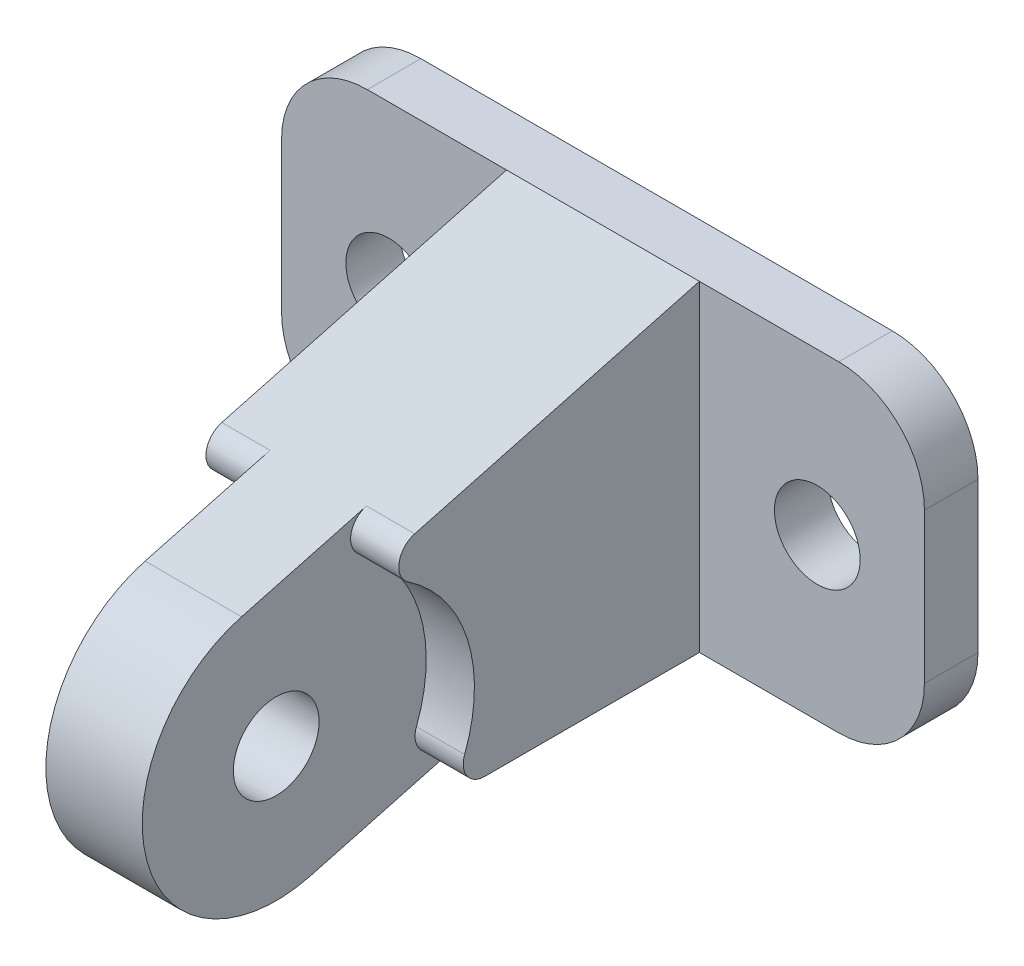
ISO-10303-21;
HEADER;
FILE_DESCRIPTION(('STEP AP214'),'2;1');
FILE_NAME('part.step','',(''),(''),'','','');
FILE_SCHEMA(('AUTOMOTIVE_DESIGN { 1 0 10303 214 1 1 1 1 }'));
ENDSEC;
DATA;
#1=APPLICATION_CONTEXT('core data for automotive mechanical design processes');
#2=APPLICATION_PROTOCOL_DEFINITION('international standard','automotive_design',2000,#1);
#3=PRODUCT_CONTEXT('',#1,'mechanical');
#4=PRODUCT('Part','Part','',(#3));
#5=PRODUCT_RELATED_PRODUCT_CATEGORY('part','',(#4));
#6=PRODUCT_DEFINITION_FORMATION('','',#4);
#7=PRODUCT_DEFINITION_CONTEXT('part definition',#1,'design');
#8=PRODUCT_DEFINITION('design','',#6,#7);
#9=PRODUCT_DEFINITION_SHAPE('','',#8);
#10=(LENGTH_UNIT() NAMED_UNIT(*) SI_UNIT(.MILLI.,.METRE.));
#11=(NAMED_UNIT(*) PLANE_ANGLE_UNIT() SI_UNIT($,.RADIAN.));
#12=(NAMED_UNIT(*) SI_UNIT($,.STERADIAN.) SOLID_ANGLE_UNIT());
#13=UNCERTAINTY_MEASURE_WITH_UNIT(LENGTH_MEASURE(1.E-05),#10,'distance_accuracy_value','');
#14=(GEOMETRIC_REPRESENTATION_CONTEXT(3) GLOBAL_UNCERTAINTY_ASSIGNED_CONTEXT((#13)) GLOBAL_UNIT_ASSIGNED_CONTEXT((#10,
#11,#12)) REPRESENTATION_CONTEXT('',''));
#15=CARTESIAN_POINT('',(0.,0.,0.));
#16=DIRECTION('',(0.,0.,1.));
#17=DIRECTION('',(1.,0.,0.));
#18=AXIS2_PLACEMENT_3D('',#15,#16,#17);
#19=CARTESIAN_POINT('',(9.,5.9476909573895,31.0562706625249));
#20=DIRECTION('',(-1.,0.,0.));
#21=DIRECTION('',(0.,0.,1.));
#22=AXIS2_PLACEMENT_3D('',#19,#20,#21);
#23=CYLINDRICAL_SURFACE('',#22,2.);
#24=CARTESIAN_POINT('',(-4.5,5.9476909573895,31.0562706625249));
#25=DIRECTION('',(1.,0.,0.));
#26=DIRECTION('',(0.,0.,-1.));
#27=AXIS2_PLACEMENT_3D('',#24,#25,#26);
#28=CIRCLE('',#27,2.);
#29=CARTESIAN_POINT('',(-4.5,7.87954260996765,31.5739087527299));
#30=VERTEX_POINT('',#29);
#31=CARTESIAN_POINT('',(-4.5,4.28933283893889,32.1742368297093));
#32=VERTEX_POINT('',#31);
#33=EDGE_CURVE('E223',#30,#32,#28,.T.);
#34=ORIENTED_EDGE('',*,*,#33,.F.);
#35=DIRECTION('',(-1.,0.,0.));
#36=VECTOR('',#35,1.);
#37=CARTESIAN_POINT('',(9.,7.87954260996765,31.5739087527299));
#38=LINE('',#37,#36);
#39=CARTESIAN_POINT('',(-9.,7.87954260996765,31.5739087527299));
#40=VERTEX_POINT('',#39);
#41=EDGE_CURVE('E292',#30,#40,#38,.T.);
#42=ORIENTED_EDGE('',*,*,#41,.T.);
#43=CARTESIAN_POINT('',(-9.,5.9476909573895,31.0562706625249));
#44=DIRECTION('',(1.,0.,0.));
#45=DIRECTION('',(0.,0.,-1.));
#46=AXIS2_PLACEMENT_3D('',#43,#44,#45);
#47=CIRCLE('',#46,2.);
#48=CARTESIAN_POINT('',(-9.,4.28933283893889,32.1742368297093));
#49=VERTEX_POINT('',#48);
#50=EDGE_CURVE('E264',#40,#49,#47,.T.);
#51=ORIENTED_EDGE('',*,*,#50,.T.);
#52=DIRECTION('',(-1.,0.,0.));
#53=VECTOR('',#52,1.);
#54=CARTESIAN_POINT('',(9.,4.28933283893889,32.1742368297093));
#55=LINE('',#54,#53);
#56=EDGE_CURVE('E290',#32,#49,#55,.T.);
#57=ORIENTED_EDGE('',*,*,#56,.F.);
#58=EDGE_LOOP('',(#34,#42,#51,#57));
#59=FACE_BOUND('',#58,.T.);
#60=ADVANCED_FACE('F41',(#59),#23,.T.);
#61=CARTESIAN_POINT('',(9.,-7.31917399021537,40.));
#62=DIRECTION('',(-1.,0.,0.));
#63=DIRECTION('',(0.,0.,1.));
#64=AXIS2_PLACEMENT_3D('',#61,#62,#63);
#65=CYLINDRICAL_SURFACE('',#64,14.);
#66=DIRECTION('',(-1.,0.,0.));
#67=VECTOR('',#66,1.);
#68=CARTESIAN_POINT('',(9.,-12.2898967487769,26.9121462700136));
#69=LINE('',#68,#67);
#70=CARTESIAN_POINT('',(-4.5,-12.2898967487769,26.9121462700136));
#71=VERTEX_POINT('',#70);
#72=CARTESIAN_POINT('',(-9.,-12.2898967487769,26.9121462700136));
#73=VERTEX_POINT('',#72);
#74=EDGE_CURVE('E284',#71,#73,#69,.T.);
#75=ORIENTED_EDGE('',*,*,#74,.F.);
#76=CARTESIAN_POINT('',(-4.5,-7.31917399021537,40.));
#77=DIRECTION('',(1.,0.,0.));
#78=DIRECTION('',(0.,0.,-1.));
#79=AXIS2_PLACEMENT_3D('',#76,#77,#78);
#80=CIRCLE('',#79,14.);
#81=EDGE_CURVE('E239',#71,#32,#80,.T.);
#82=ORIENTED_EDGE('',*,*,#81,.T.);
#83=ORIENTED_EDGE('',*,*,#56,.T.);
#84=CARTESIAN_POINT('',(-9.,-7.31917399021537,40.));
#85=DIRECTION('',(1.,0.,0.));
#86=DIRECTION('',(0.,0.,-1.));
#87=AXIS2_PLACEMENT_3D('',#84,#85,#86);
#88=CIRCLE('',#87,14.);
#89=EDGE_CURVE('E268',#73,#49,#88,.T.);
#90=ORIENTED_EDGE('',*,*,#89,.F.);
#91=EDGE_LOOP('',(#75,#82,#83,#90));
#92=FACE_BOUND('',#91,.T.);
#93=ADVANCED_FACE('F445',(#92),#65,.F.);
#94=CARTESIAN_POINT('',(9.,-13.,25.0424528800156));
#95=DIRECTION('',(-1.,0.,0.));
#96=DIRECTION('',(0.,0.,1.));
#97=AXIS2_PLACEMENT_3D('',#94,#95,#96);
#98=CYLINDRICAL_SURFACE('',#97,2.);
#99=CARTESIAN_POINT('',(-4.5,-13.,25.0424528800156));
#100=DIRECTION('',(1.,0.,0.));
#101=DIRECTION('',(0.,0.,-1.));
#102=AXIS2_PLACEMENT_3D('',#99,#100,#101);
#103=CIRCLE('',#102,2.);
#104=CARTESIAN_POINT('',(-4.5,-15.,25.0424528800156));
#105=VERTEX_POINT('',#104);
#106=EDGE_CURVE('E237',#71,#105,#103,.T.);
#107=ORIENTED_EDGE('',*,*,#106,.F.);
#108=ORIENTED_EDGE('',*,*,#74,.T.);
#109=CARTESIAN_POINT('',(-9.,-13.,25.0424528800156));
#110=DIRECTION('',(1.,0.,0.));
#111=DIRECTION('',(0.,0.,-1.));
#112=AXIS2_PLACEMENT_3D('',#109,#110,#111);
#113=CIRCLE('',#112,2.);
#114=CARTESIAN_POINT('',(-9.,-15.,25.0424528800156));
#115=VERTEX_POINT('',#114);
#116=EDGE_CURVE('E271',#73,#115,#113,.T.);
#117=ORIENTED_EDGE('',*,*,#116,.T.);
#118=DIRECTION('',(-1.,0.,0.));
#119=VECTOR('',#118,1.);
#120=CARTESIAN_POINT('',(9.,-15.,25.0424528800156));
#121=LINE('',#120,#119);
#122=EDGE_CURVE('E278',#105,#115,#121,.T.);
#123=ORIENTED_EDGE('',*,*,#122,.F.);
#124=EDGE_LOOP('',(#107,#108,#117,#123));
#125=FACE_BOUND('',#124,.T.);
#126=ADVANCED_FACE('F409',(#125),#98,.T.);
#127=CARTESIAN_POINT('',(-22.,-7.,5.));
#128=DIRECTION('',(0.,0.,-1.));
#129=DIRECTION('',(-1.,0.,0.));
#130=AXIS2_PLACEMENT_3D('',#127,#128,#129);
#131=PLANE('',#130);
#132=CARTESIAN_POINT('',(-20.,0.,5.));
#133=DIRECTION('',(0.,0.,1.));
#134=DIRECTION('',(1.,0.,0.));
#135=AXIS2_PLACEMENT_3D('',#132,#133,#134);
#136=CIRCLE('',#135,4.);
#137=CARTESIAN_POINT('',(-16.,0.,5.));
#138=VERTEX_POINT('',#137);
#139=EDGE_CURVE('E293',#138,#138,#136,.T.);
#140=ORIENTED_EDGE('',*,*,#139,.F.);
#141=EDGE_LOOP('',(#140));
#142=FACE_BOUND('',#141,.T.);
#143=DIRECTION('',(0.,-1.,0.));
#144=VECTOR('',#143,1.);
#145=CARTESIAN_POINT('',(-9.,0.,5.));
#146=LINE('',#145,#144);
#147=CARTESIAN_POINT('',(-9.,15.,5.));
#148=VERTEX_POINT('',#147);
#149=CARTESIAN_POINT('',(-9.,-15.,5.));
#150=VERTEX_POINT('',#149);
#151=EDGE_CURVE('E248',#148,#150,#146,.T.);
#152=ORIENTED_EDGE('',*,*,#151,.F.);
#153=DIRECTION('',(-1.,0.,0.));
#154=VECTOR('',#153,1.);
#155=CARTESIAN_POINT('',(-21.9999999999999,15.,5.));
#156=LINE('',#155,#154);
#157=CARTESIAN_POINT('',(-21.9999999999999,15.,5.));
#158=VERTEX_POINT('',#157);
#159=EDGE_CURVE('E321',#148,#158,#156,.T.);
#160=ORIENTED_EDGE('',*,*,#159,.T.);
#161=CARTESIAN_POINT('',(-22.,7.,5.));
#162=DIRECTION('',(0.,0.,1.));
#163=DIRECTION('',(-1.,0.,0.));
#164=AXIS2_PLACEMENT_3D('',#161,#162,#163);
#165=CIRCLE('',#164,8.);
#166=CARTESIAN_POINT('',(-30.,6.99999999999994,5.));
#167=VERTEX_POINT('',#166);
#168=EDGE_CURVE('E324',#158,#167,#165,.T.);
#169=ORIENTED_EDGE('',*,*,#168,.T.);
#170=DIRECTION('',(0.,-1.,0.));
#171=VECTOR('',#170,1.);
#172=CARTESIAN_POINT('',(-30.,-6.99999999999994,5.));
#173=LINE('',#172,#171);
#174=CARTESIAN_POINT('',(-30.,-6.99999999999994,5.));
#175=VERTEX_POINT('',#174);
#176=EDGE_CURVE('E330',#167,#175,#173,.T.);
#177=ORIENTED_EDGE('',*,*,#176,.T.);
#178=CARTESIAN_POINT('',(-22.,-7.,5.));
#179=DIRECTION('',(0.,0.,1.));
#180=DIRECTION('',(-1.,0.,0.));
#181=AXIS2_PLACEMENT_3D('',#178,#179,#180);
#182=CIRCLE('',#181,8.);
#183=CARTESIAN_POINT('',(-21.9999999999999,-15.,5.));
#184=VERTEX_POINT('',#183);
#185=EDGE_CURVE('E307',#175,#184,#182,.T.);
#186=ORIENTED_EDGE('',*,*,#185,.T.);
#187=DIRECTION('',(1.,0.,0.));
#188=VECTOR('',#187,1.);
#189=CARTESIAN_POINT('',(-21.9999999999999,-15.,5.));
#190=LINE('',#189,#188);
#191=EDGE_CURVE('E315',#184,#150,#190,.T.);
#192=ORIENTED_EDGE('',*,*,#191,.T.);
#193=EDGE_LOOP('',(#152,#160,#169,#177,#186,#192));
#194=FACE_BOUND('',#193,.T.);
#195=ADVANCED_FACE('F416',(#142,#194),#131,.F.);
#196=CARTESIAN_POINT('',(21.9999999999999,15.,5.));
#197=VERTEX_POINT('',#196);
#198=CARTESIAN_POINT('',(9.,15.,5.));
#199=VERTEX_POINT('',#198);
#200=EDGE_CURVE('E325',#197,#199,#156,.T.);
#201=ORIENTED_EDGE('',*,*,#200,.T.);
#202=DIRECTION('',(0.,-1.,0.));
#203=VECTOR('',#202,1.);
#204=CARTESIAN_POINT('',(9.,0.,5.));
#205=LINE('',#204,#203);
#206=CARTESIAN_POINT('',(9.,-15.,5.));
#207=VERTEX_POINT('',#206);
#208=EDGE_CURVE('E257',#199,#207,#205,.T.);
#209=ORIENTED_EDGE('',*,*,#208,.T.);
#210=CARTESIAN_POINT('',(21.9999999999999,-15.,5.));
#211=VERTEX_POINT('',#210);
#212=EDGE_CURVE('E309',#207,#211,#190,.T.);
#213=ORIENTED_EDGE('',*,*,#212,.T.);
#214=CARTESIAN_POINT('',(22.,-7.,5.));
#215=DIRECTION('',(0.,0.,1.));
#216=DIRECTION('',(1.,0.,0.));
#217=AXIS2_PLACEMENT_3D('',#214,#215,#216);
#218=CIRCLE('',#217,8.);
#219=CARTESIAN_POINT('',(30.,-7.,5.));
#220=VERTEX_POINT('',#219);
#221=EDGE_CURVE('E312',#211,#220,#218,.T.);
#222=ORIENTED_EDGE('',*,*,#221,.T.);
#223=DIRECTION('',(0.,1.,0.));
#224=VECTOR('',#223,1.);
#225=CARTESIAN_POINT('',(30.,-6.99999999999994,5.));
#226=LINE('',#225,#224);
#227=CARTESIAN_POINT('',(30.,6.99999999999994,5.));
#228=VERTEX_POINT('',#227);
#229=EDGE_CURVE('E320',#220,#228,#226,.T.);
#230=ORIENTED_EDGE('',*,*,#229,.T.);
#231=CARTESIAN_POINT('',(22.,7.,5.));
#232=DIRECTION('',(0.,0.,1.));
#233=DIRECTION('',(-1.,0.,0.));
#234=AXIS2_PLACEMENT_3D('',#231,#232,#233);
#235=CIRCLE('',#234,8.);
#236=EDGE_CURVE('E317',#228,#197,#235,.T.);
#237=ORIENTED_EDGE('',*,*,#236,.T.);
#238=EDGE_LOOP('',(#201,#209,#213,#222,#230,#237));
#239=FACE_BOUND('',#238,.T.);
#240=CARTESIAN_POINT('',(20.,0.,5.));
#241=DIRECTION('',(0.,0.,1.));
#242=DIRECTION('',(1.,0.,0.));
#243=AXIS2_PLACEMENT_3D('',#240,#241,#242);
#244=CIRCLE('',#243,4.);
#245=CARTESIAN_POINT('',(24.,0.,5.));
#246=VERTEX_POINT('',#245);
#247=EDGE_CURVE('E302',#246,#246,#244,.T.);
#248=ORIENTED_EDGE('',*,*,#247,.F.);
#249=EDGE_LOOP('',(#248));
#250=FACE_BOUND('',#249,.T.);
#251=ADVANCED_FACE('F387',(#239,#250),#131,.F.);
#252=CARTESIAN_POINT('',(-22.,-7.,0.));
#253=DIRECTION('',(0.,0.,-1.));
#254=DIRECTION('',(-1.,0.,0.));
#255=AXIS2_PLACEMENT_3D('',#252,#253,#254);
#256=PLANE('',#255);
#257=CARTESIAN_POINT('',(20.,0.,0.));
#258=DIRECTION('',(0.,0.,1.));
#259=DIRECTION('',(1.,0.,0.));
#260=AXIS2_PLACEMENT_3D('',#257,#258,#259);
#261=CIRCLE('',#260,4.);
#262=CARTESIAN_POINT('',(24.,0.,0.));
#263=VERTEX_POINT('',#262);
#264=EDGE_CURVE('E299',#263,#263,#261,.T.);
#265=ORIENTED_EDGE('',*,*,#264,.T.);
#266=EDGE_LOOP('',(#265));
#267=FACE_BOUND('',#266,.T.);
#268=CARTESIAN_POINT('',(-22.,-7.,0.));
#269=DIRECTION('',(0.,0.,1.));
#270=DIRECTION('',(-1.,0.,0.));
#271=AXIS2_PLACEMENT_3D('',#268,#269,#270);
#272=CIRCLE('',#271,8.);
#273=CARTESIAN_POINT('',(-30.,-6.99999999999994,0.));
#274=VERTEX_POINT('',#273);
#275=CARTESIAN_POINT('',(-21.9999999999999,-15.,0.));
#276=VERTEX_POINT('',#275);
#277=EDGE_CURVE('E301',#274,#276,#272,.T.);
#278=ORIENTED_EDGE('',*,*,#277,.F.);
#279=DIRECTION('',(0.,-1.,0.));
#280=VECTOR('',#279,1.);
#281=CARTESIAN_POINT('',(-30.,-6.99999999999994,0.));
#282=LINE('',#281,#280);
#283=CARTESIAN_POINT('',(-30.,6.99999999999994,0.));
#284=VERTEX_POINT('',#283);
#285=EDGE_CURVE('E313',#284,#274,#282,.T.);
#286=ORIENTED_EDGE('',*,*,#285,.F.);
#287=CARTESIAN_POINT('',(-22.,7.,0.));
#288=DIRECTION('',(0.,0.,1.));
#289=DIRECTION('',(-1.,0.,0.));
#290=AXIS2_PLACEMENT_3D('',#287,#288,#289);
#291=CIRCLE('',#290,8.);
#292=CARTESIAN_POINT('',(-21.9999999999999,15.,0.));
#293=VERTEX_POINT('',#292);
#294=EDGE_CURVE('E345',#293,#284,#291,.T.);
#295=ORIENTED_EDGE('',*,*,#294,.F.);
#296=DIRECTION('',(-1.,0.,0.));
#297=VECTOR('',#296,1.);
#298=CARTESIAN_POINT('',(-21.9999999999999,15.,0.));
#299=LINE('',#298,#297);
#300=CARTESIAN_POINT('',(21.9999999999999,15.,0.));
#301=VERTEX_POINT('',#300);
#302=EDGE_CURVE('E340',#301,#293,#299,.T.);
#303=ORIENTED_EDGE('',*,*,#302,.F.);
#304=CARTESIAN_POINT('',(22.,7.,0.));
#305=DIRECTION('',(0.,0.,1.));
#306=DIRECTION('',(-1.,0.,0.));
#307=AXIS2_PLACEMENT_3D('',#304,#305,#306);
#308=CIRCLE('',#307,8.);
#309=CARTESIAN_POINT('',(30.,6.99999999999994,0.));
#310=VERTEX_POINT('',#309);
#311=EDGE_CURVE('E339',#310,#301,#308,.T.);
#312=ORIENTED_EDGE('',*,*,#311,.F.);
#313=DIRECTION('',(0.,1.,0.));
#314=VECTOR('',#313,1.);
#315=CARTESIAN_POINT('',(30.,-6.99999999999994,0.));
#316=LINE('',#315,#314);
#317=CARTESIAN_POINT('',(30.,-7.,0.));
#318=VERTEX_POINT('',#317);
#319=EDGE_CURVE('E336',#318,#310,#316,.T.);
#320=ORIENTED_EDGE('',*,*,#319,.F.);
#321=CARTESIAN_POINT('',(22.,-7.,0.));
#322=DIRECTION('',(0.,0.,1.));
#323=DIRECTION('',(1.,0.,0.));
#324=AXIS2_PLACEMENT_3D('',#321,#322,#323);
#325=CIRCLE('',#324,8.);
#326=CARTESIAN_POINT('',(21.9999999999999,-15.,0.));
#327=VERTEX_POINT('',#326);
#328=EDGE_CURVE('E331',#327,#318,#325,.T.);
#329=ORIENTED_EDGE('',*,*,#328,.F.);
#330=DIRECTION('',(1.,0.,0.));
#331=VECTOR('',#330,1.);
#332=CARTESIAN_POINT('',(-21.9999999999999,-15.,0.));
#333=LINE('',#332,#331);
#334=EDGE_CURVE('E335',#276,#327,#333,.T.);
#335=ORIENTED_EDGE('',*,*,#334,.F.);
#336=EDGE_LOOP('',(#278,#286,#295,#303,#312,#320,#329,#335));
#337=FACE_BOUND('',#336,.T.);
#338=CARTESIAN_POINT('',(-20.,0.,0.));
#339=DIRECTION('',(0.,0.,1.));
#340=DIRECTION('',(1.,0.,0.));
#341=AXIS2_PLACEMENT_3D('',#338,#339,#340);
#342=CIRCLE('',#341,4.);
#343=CARTESIAN_POINT('',(-16.,0.,0.));
#344=VERTEX_POINT('',#343);
#345=EDGE_CURVE('E294',#344,#344,#342,.T.);
#346=ORIENTED_EDGE('',*,*,#345,.T.);
#347=EDGE_LOOP('',(#346));
#348=FACE_BOUND('',#347,.T.);
#349=ADVANCED_FACE('F375',(#267,#337,#348),#256,.T.);
#350=CARTESIAN_POINT('',(-22.,-7.,5.));
#351=DIRECTION('',(0.,0.,-1.));
#352=DIRECTION('',(-1.,0.,0.));
#353=AXIS2_PLACEMENT_3D('',#350,#351,#352);
#354=CYLINDRICAL_SURFACE('',#353,8.);
#355=ORIENTED_EDGE('',*,*,#277,.T.);
#356=DIRECTION('',(0.,0.,-1.));
#357=VECTOR('',#356,1.);
#358=CARTESIAN_POINT('',(-21.9999999999999,-15.,5.));
#359=LINE('',#358,#357);
#360=EDGE_CURVE('E11',#184,#276,#359,.T.);
#361=ORIENTED_EDGE('',*,*,#360,.F.);
#362=ORIENTED_EDGE('',*,*,#185,.F.);
#363=DIRECTION('',(0.,0.,-1.));
#364=VECTOR('',#363,1.);
#365=CARTESIAN_POINT('',(-30.,-6.99999999999994,5.));
#366=LINE('',#365,#364);
#367=EDGE_CURVE('E328',#175,#274,#366,.T.);
#368=ORIENTED_EDGE('',*,*,#367,.T.);
#369=EDGE_LOOP('',(#355,#361,#362,#368));
#370=FACE_BOUND('',#369,.T.);
#371=ADVANCED_FACE('F43',(#370),#354,.T.);
#372=CARTESIAN_POINT('',(-21.9999999999999,-15.,5.));
#373=DIRECTION('',(0.,1.,0.));
#374=DIRECTION('',(0.,0.,1.));
#375=AXIS2_PLACEMENT_3D('',#372,#373,#374);
#376=PLANE('',#375);
#377=CARTESIAN_POINT('',(9.,-15.,25.0424528800156));
#378=VERTEX_POINT('',#377);
#379=CARTESIAN_POINT('',(4.5,-15.,25.0424528800156));
#380=VERTEX_POINT('',#379);
#381=EDGE_CURVE('E281',#378,#380,#121,.T.);
#382=ORIENTED_EDGE('',*,*,#381,.T.);
#383=DIRECTION('',(0.,0.,1.));
#384=VECTOR('',#383,1.);
#385=CARTESIAN_POINT('',(4.5,-15.,0.));
#386=LINE('',#385,#384);
#387=CARTESIAN_POINT('',(4.5,-15.,20.3704918261027));
#388=VERTEX_POINT('',#387);
#389=EDGE_CURVE('E57',#388,#380,#386,.T.);
#390=ORIENTED_EDGE('',*,*,#389,.F.);
#391=DIRECTION('',(-1.,0.,0.));
#392=VECTOR('',#391,1.);
#393=CARTESIAN_POINT('',(4.5,-15.,20.3704918261027));
#394=LINE('',#393,#392);
#395=CARTESIAN_POINT('',(-4.5,-15.,20.3704918261027));
#396=VERTEX_POINT('',#395);
#397=EDGE_CURVE('E58',#388,#396,#394,.T.);
#398=ORIENTED_EDGE('',*,*,#397,.T.);
#399=DIRECTION('',(0.,0.,1.));
#400=VECTOR('',#399,1.);
#401=CARTESIAN_POINT('',(-4.5,-15.,0.));
#402=LINE('',#401,#400);
#403=EDGE_CURVE('E231',#396,#105,#402,.T.);
#404=ORIENTED_EDGE('',*,*,#403,.T.);
#405=ORIENTED_EDGE('',*,*,#122,.T.);
#406=DIRECTION('',(0.,0.,1.));
#407=VECTOR('',#406,1.);
#408=CARTESIAN_POINT('',(-9.,-15.,0.));
#409=LINE('',#408,#407);
#410=EDGE_CURVE('E273',#150,#115,#409,.T.);
#411=ORIENTED_EDGE('',*,*,#410,.F.);
#412=ORIENTED_EDGE('',*,*,#191,.F.);
#413=ORIENTED_EDGE('',*,*,#360,.T.);
#414=ORIENTED_EDGE('',*,*,#334,.T.);
#415=DIRECTION('',(0.,0.,-1.));
#416=VECTOR('',#415,1.);
#417=CARTESIAN_POINT('',(21.9999999999999,-15.,5.));
#418=LINE('',#417,#416);
#419=EDGE_CURVE('E47',#211,#327,#418,.T.);
#420=ORIENTED_EDGE('',*,*,#419,.F.);
#421=ORIENTED_EDGE('',*,*,#212,.F.);
#422=DIRECTION('',(0.,0.,1.));
#423=VECTOR('',#422,1.);
#424=CARTESIAN_POINT('',(9.,-15.,0.));
#425=LINE('',#424,#423);
#426=EDGE_CURVE('E260',#207,#378,#425,.T.);
#427=ORIENTED_EDGE('',*,*,#426,.T.);
#428=EDGE_LOOP('',(#382,#390,#398,#404,#405,#411,#412,#413,#414,#420,#421,#427));
#429=FACE_BOUND('',#428,.T.);
#430=ADVANCED_FACE('F386',(#429),#376,.F.);
#431=CARTESIAN_POINT('',(22.,-7.,5.));
#432=DIRECTION('',(0.,0.,-1.));
#433=DIRECTION('',(-1.,0.,0.));
#434=AXIS2_PLACEMENT_3D('',#431,#432,#433);
#435=CYLINDRICAL_SURFACE('',#434,8.);
#436=ORIENTED_EDGE('',*,*,#328,.T.);
#437=DIRECTION('',(0.,0.,-1.));
#438=VECTOR('',#437,1.);
#439=CARTESIAN_POINT('',(30.,-7.,5.));
#440=LINE('',#439,#438);
#441=EDGE_CURVE('E356',#220,#318,#440,.T.);
#442=ORIENTED_EDGE('',*,*,#441,.F.);
#443=ORIENTED_EDGE('',*,*,#221,.F.);
#444=ORIENTED_EDGE('',*,*,#419,.T.);
#445=EDGE_LOOP('',(#436,#442,#443,#444));
#446=FACE_BOUND('',#445,.T.);
#447=ADVANCED_FACE('F368',(#446),#435,.T.);
#448=CARTESIAN_POINT('',(30.,-6.99999999999994,5.));
#449=DIRECTION('',(-1.,0.,0.));
#450=DIRECTION('',(0.,0.,1.));
#451=AXIS2_PLACEMENT_3D('',#448,#449,#450);
#452=PLANE('',#451);
#453=ORIENTED_EDGE('',*,*,#319,.T.);
#454=DIRECTION('',(0.,0.,-1.));
#455=VECTOR('',#454,1.);
#456=CARTESIAN_POINT('',(30.,6.99999999999994,5.));
#457=LINE('',#456,#455);
#458=EDGE_CURVE('E357',#228,#310,#457,.T.);
#459=ORIENTED_EDGE('',*,*,#458,.F.);
#460=ORIENTED_EDGE('',*,*,#229,.F.);
#461=ORIENTED_EDGE('',*,*,#441,.T.);
#462=EDGE_LOOP('',(#453,#459,#460,#461));
#463=FACE_BOUND('',#462,.T.);
#464=ADVANCED_FACE('F378',(#463),#452,.F.);
#465=CARTESIAN_POINT('',(22.,7.,5.));
#466=DIRECTION('',(0.,0.,-1.));
#467=DIRECTION('',(-1.,0.,0.));
#468=AXIS2_PLACEMENT_3D('',#465,#466,#467);
#469=CYLINDRICAL_SURFACE('',#468,8.);
#470=ORIENTED_EDGE('',*,*,#311,.T.);
#471=DIRECTION('',(0.,0.,-1.));
#472=VECTOR('',#471,1.);
#473=CARTESIAN_POINT('',(21.9999999999999,15.,5.));
#474=LINE('',#473,#472);
#475=EDGE_CURVE('E354',#197,#301,#474,.T.);
#476=ORIENTED_EDGE('',*,*,#475,.F.);
#477=ORIENTED_EDGE('',*,*,#236,.F.);
#478=ORIENTED_EDGE('',*,*,#458,.T.);
#479=EDGE_LOOP('',(#470,#476,#477,#478));
#480=FACE_BOUND('',#479,.T.);
#481=ADVANCED_FACE('F385',(#480),#469,.T.);
#482=CARTESIAN_POINT('',(-21.9999999999999,15.,5.));
#483=DIRECTION('',(0.,-1.,0.));
#484=DIRECTION('',(0.,0.,-1.));
#485=AXIS2_PLACEMENT_3D('',#482,#483,#484);
#486=PLANE('',#485);
#487=ORIENTED_EDGE('',*,*,#302,.T.);
#488=DIRECTION('',(0.,0.,-1.));
#489=VECTOR('',#488,1.);
#490=CARTESIAN_POINT('',(-21.9999999999999,15.,5.));
#491=LINE('',#490,#489);
#492=EDGE_CURVE('E348',#158,#293,#491,.T.);
#493=ORIENTED_EDGE('',*,*,#492,.F.);
#494=ORIENTED_EDGE('',*,*,#159,.F.);
#495=DIRECTION('',(-1.,0.,0.));
#496=VECTOR('',#495,1.);
#497=CARTESIAN_POINT('',(9.,15.,5.));
#498=LINE('',#497,#496);
#499=EDGE_CURVE('E263',#199,#148,#498,.T.);
#500=ORIENTED_EDGE('',*,*,#499,.F.);
#501=ORIENTED_EDGE('',*,*,#200,.F.);
#502=ORIENTED_EDGE('',*,*,#475,.T.);
#503=EDGE_LOOP('',(#487,#493,#494,#500,#501,#502));
#504=FACE_BOUND('',#503,.T.);
#505=ADVANCED_FACE('F432',(#504),#486,.F.);
#506=CARTESIAN_POINT('',(-22.,7.,5.));
#507=DIRECTION('',(0.,0.,-1.));
#508=DIRECTION('',(-1.,0.,0.));
#509=AXIS2_PLACEMENT_3D('',#506,#507,#508);
#510=CYLINDRICAL_SURFACE('',#509,8.);
#511=ORIENTED_EDGE('',*,*,#294,.T.);
#512=DIRECTION('',(0.,0.,-1.));
#513=VECTOR('',#512,1.);
#514=CARTESIAN_POINT('',(-30.,6.99999999999994,5.));
#515=LINE('',#514,#513);
#516=EDGE_CURVE('E350',#167,#284,#515,.T.);
#517=ORIENTED_EDGE('',*,*,#516,.F.);
#518=ORIENTED_EDGE('',*,*,#168,.F.);
#519=ORIENTED_EDGE('',*,*,#492,.T.);
#520=EDGE_LOOP('',(#511,#517,#518,#519));
#521=FACE_BOUND('',#520,.T.);
#522=ADVANCED_FACE('F431',(#521),#510,.T.);
#523=CARTESIAN_POINT('',(-30.,-6.99999999999994,5.));
#524=DIRECTION('',(1.,0.,0.));
#525=DIRECTION('',(0.,0.,-1.));
#526=AXIS2_PLACEMENT_3D('',#523,#524,#525);
#527=PLANE('',#526);
#528=ORIENTED_EDGE('',*,*,#285,.T.);
#529=ORIENTED_EDGE('',*,*,#367,.F.);
#530=ORIENTED_EDGE('',*,*,#176,.F.);
#531=ORIENTED_EDGE('',*,*,#516,.T.);
#532=EDGE_LOOP('',(#528,#529,#530,#531));
#533=FACE_BOUND('',#532,.T.);
#534=ADVANCED_FACE('F426',(#533),#527,.F.);
#535=CARTESIAN_POINT('',(20.,0.,5.));
#536=DIRECTION('',(0.,0.,-1.));
#537=DIRECTION('',(-1.,0.,0.));
#538=AXIS2_PLACEMENT_3D('',#535,#536,#537);
#539=CYLINDRICAL_SURFACE('',#538,4.);
#540=ORIENTED_EDGE('',*,*,#247,.T.);
#541=EDGE_LOOP('',(#540));
#542=FACE_BOUND('',#541,.T.);
#543=ORIENTED_EDGE('',*,*,#264,.F.);
#544=EDGE_LOOP('',(#543));
#545=FACE_BOUND('',#544,.T.);
#546=ADVANCED_FACE('F461',(#542,#545),#539,.F.);
#547=CARTESIAN_POINT('',(-20.,0.,5.));
#548=DIRECTION('',(0.,0.,-1.));
#549=DIRECTION('',(-1.,0.,0.));
#550=AXIS2_PLACEMENT_3D('',#547,#548,#549);
#551=CYLINDRICAL_SURFACE('',#550,4.);
#552=ORIENTED_EDGE('',*,*,#139,.T.);
#553=EDGE_LOOP('',(#552));
#554=FACE_BOUND('',#553,.T.);
#555=ORIENTED_EDGE('',*,*,#345,.F.);
#556=EDGE_LOOP('',(#555));
#557=FACE_BOUND('',#556,.T.);
#558=ADVANCED_FACE('F459',(#554,#557),#551,.F.);
#559=CARTESIAN_POINT('',(9.,15.2451905283833,4.08493649053891));
#560=DIRECTION('',(0.,-0.965925826289068,-0.258819045102521));
#561=DIRECTION('',(0.,0.258819045102521,-0.965925826289068));
#562=AXIS2_PLACEMENT_3D('',#559,#560,#561);
#563=PLANE('',#562);
#564=DIRECTION('',(0.,-0.258819045102521,0.965925826289068));
#565=VECTOR('',#564,1.);
#566=CARTESIAN_POINT('',(-9.,15.2451905283833,4.08493649053891));
#567=LINE('',#566,#565);
#568=EDGE_CURVE('E210',#148,#40,#567,.T.);
#569=ORIENTED_EDGE('',*,*,#568,.T.);
#570=ORIENTED_EDGE('',*,*,#41,.F.);
#571=DIRECTION('',(0.,-0.258819045102521,0.965925826289068));
#572=VECTOR('',#571,1.);
#573=CARTESIAN_POINT('',(-4.5,15.2451905283833,4.08493649053891));
#574=LINE('',#573,#572);
#575=CARTESIAN_POINT('',(-4.5,4.75489883839799,43.2352380637815));
#576=VERTEX_POINT('',#575);
#577=EDGE_CURVE('E201',#30,#576,#574,.T.);
#578=ORIENTED_EDGE('',*,*,#577,.T.);
#579=DIRECTION('',(-1.,0.,0.));
#580=VECTOR('',#579,1.);
#581=CARTESIAN_POINT('',(4.5,4.75489883839799,43.2352380637815));
#582=LINE('',#581,#580);
#583=CARTESIAN_POINT('',(4.5,4.75489883839799,43.2352380637815));
#584=VERTEX_POINT('',#583);
#585=EDGE_CURVE('E196',#584,#576,#582,.T.);
#586=ORIENTED_EDGE('',*,*,#585,.F.);
#587=DIRECTION('',(0.,-0.258819045102521,0.965925826289068));
#588=VECTOR('',#587,1.);
#589=CARTESIAN_POINT('',(4.5,15.2451905283833,4.08493649053891));
#590=LINE('',#589,#588);
#591=CARTESIAN_POINT('',(4.5,7.87954260996765,31.5739087527299));
#592=VERTEX_POINT('',#591);
#593=EDGE_CURVE('E184',#592,#584,#590,.T.);
#594=ORIENTED_EDGE('',*,*,#593,.F.);
#595=CARTESIAN_POINT('',(9.,7.87954260996765,31.5739087527299));
#596=VERTEX_POINT('',#595);
#597=EDGE_CURVE('E295',#596,#592,#38,.T.);
#598=ORIENTED_EDGE('',*,*,#597,.F.);
#599=DIRECTION('',(0.,-0.258819045102521,0.965925826289068));
#600=VECTOR('',#599,1.);
#601=CARTESIAN_POINT('',(9.,15.2451905283833,4.08493649053891));
#602=LINE('',#601,#600);
#603=EDGE_CURVE('E247',#199,#596,#602,.T.);
#604=ORIENTED_EDGE('',*,*,#603,.F.);
#605=ORIENTED_EDGE('',*,*,#499,.T.);
#606=EDGE_LOOP('',(#569,#570,#578,#586,#594,#598,#604,#605));
#607=FACE_BOUND('',#606,.T.);
#608=ADVANCED_FACE('F199',(#607),#563,.F.);
#609=ORIENTED_EDGE('',*,*,#597,.T.);
#610=CARTESIAN_POINT('',(4.5,5.9476909573895,31.0562706625249));
#611=DIRECTION('',(1.,0.,0.));
#612=DIRECTION('',(0.,0.,-1.));
#613=AXIS2_PLACEMENT_3D('',#610,#611,#612);
#614=CIRCLE('',#613,2.);
#615=CARTESIAN_POINT('',(4.5,4.28933283893889,32.1742368297093));
#616=VERTEX_POINT('',#615);
#617=EDGE_CURVE('E194',#592,#616,#614,.T.);
#618=ORIENTED_EDGE('',*,*,#617,.T.);
#619=CARTESIAN_POINT('',(9.,4.28933283893889,32.1742368297093));
#620=VERTEX_POINT('',#619);
#621=EDGE_CURVE('E289',#620,#616,#55,.T.);
#622=ORIENTED_EDGE('',*,*,#621,.F.);
#623=CARTESIAN_POINT('',(9.,5.9476909573895,31.0562706625249));
#624=DIRECTION('',(1.,0.,0.));
#625=DIRECTION('',(0.,0.,-1.));
#626=AXIS2_PLACEMENT_3D('',#623,#624,#625);
#627=CIRCLE('',#626,2.);
#628=EDGE_CURVE('E246',#596,#620,#627,.T.);
#629=ORIENTED_EDGE('',*,*,#628,.F.);
#630=EDGE_LOOP('',(#609,#618,#622,#629));
#631=FACE_BOUND('',#630,.T.);
#632=ADVANCED_FACE('F440',(#631),#23,.T.);
#633=CARTESIAN_POINT('',(4.5,-7.31917399021537,40.));
#634=DIRECTION('',(1.,0.,0.));
#635=DIRECTION('',(0.,0.,-1.));
#636=AXIS2_PLACEMENT_3D('',#633,#634,#635);
#637=CIRCLE('',#636,14.);
#638=CARTESIAN_POINT('',(4.5,-12.2898967487769,26.9121462700136));
#639=VERTEX_POINT('',#638);
#640=EDGE_CURVE('E219',#639,#616,#637,.T.);
#641=ORIENTED_EDGE('',*,*,#640,.F.);
#642=CARTESIAN_POINT('',(9.,-12.2898967487769,26.9121462700136));
#643=VERTEX_POINT('',#642);
#644=EDGE_CURVE('E283',#643,#639,#69,.T.);
#645=ORIENTED_EDGE('',*,*,#644,.F.);
#646=CARTESIAN_POINT('',(9.,-7.31917399021537,40.));
#647=DIRECTION('',(1.,0.,0.));
#648=DIRECTION('',(0.,0.,-1.));
#649=AXIS2_PLACEMENT_3D('',#646,#647,#648);
#650=CIRCLE('',#649,14.);
#651=EDGE_CURVE('E252',#643,#620,#650,.T.);
#652=ORIENTED_EDGE('',*,*,#651,.T.);
#653=ORIENTED_EDGE('',*,*,#621,.T.);
#654=EDGE_LOOP('',(#641,#645,#652,#653));
#655=FACE_BOUND('',#654,.T.);
#656=ADVANCED_FACE('F438',(#655),#65,.F.);
#657=ORIENTED_EDGE('',*,*,#644,.T.);
#658=CARTESIAN_POINT('',(4.5,-13.,25.0424528800156));
#659=DIRECTION('',(1.,0.,0.));
#660=DIRECTION('',(0.,0.,-1.));
#661=AXIS2_PLACEMENT_3D('',#658,#659,#660);
#662=CIRCLE('',#661,2.);
#663=EDGE_CURVE('E217',#639,#380,#662,.T.);
#664=ORIENTED_EDGE('',*,*,#663,.T.);
#665=ORIENTED_EDGE('',*,*,#381,.F.);
#666=CARTESIAN_POINT('',(9.,-13.,25.0424528800156));
#667=DIRECTION('',(1.,0.,0.));
#668=DIRECTION('',(0.,0.,-1.));
#669=AXIS2_PLACEMENT_3D('',#666,#667,#668);
#670=CIRCLE('',#669,2.);
#671=EDGE_CURVE('E254',#643,#378,#670,.T.);
#672=ORIENTED_EDGE('',*,*,#671,.F.);
#673=EDGE_LOOP('',(#657,#664,#665,#672));
#674=FACE_BOUND('',#673,.T.);
#675=ADVANCED_FACE('F400',(#674),#98,.T.);
#676=CARTESIAN_POINT('',(9.,0.,0.));
#677=DIRECTION('',(1.,0.,0.));
#678=DIRECTION('',(0.,0.,-1.));
#679=AXIS2_PLACEMENT_3D('',#676,#677,#678);
#680=PLANE('',#679);
#681=ORIENTED_EDGE('',*,*,#603,.T.);
#682=ORIENTED_EDGE('',*,*,#628,.T.);
#683=ORIENTED_EDGE('',*,*,#651,.F.);
#684=ORIENTED_EDGE('',*,*,#671,.T.);
#685=ORIENTED_EDGE('',*,*,#426,.F.);
#686=ORIENTED_EDGE('',*,*,#208,.F.);
#687=EDGE_LOOP('',(#681,#682,#683,#684,#685,#686));
#688=FACE_BOUND('',#687,.T.);
#689=ADVANCED_FACE('F392',(#688),#680,.T.);
#690=CARTESIAN_POINT('',(-9.,0.,0.));
#691=DIRECTION('',(1.,0.,0.));
#692=DIRECTION('',(0.,0.,-1.));
#693=AXIS2_PLACEMENT_3D('',#690,#691,#692);
#694=PLANE('',#693);
#695=ORIENTED_EDGE('',*,*,#568,.F.);
#696=ORIENTED_EDGE('',*,*,#151,.T.);
#697=ORIENTED_EDGE('',*,*,#410,.T.);
#698=ORIENTED_EDGE('',*,*,#116,.F.);
#699=ORIENTED_EDGE('',*,*,#89,.T.);
#700=ORIENTED_EDGE('',*,*,#50,.F.);
#701=EDGE_LOOP('',(#695,#696,#697,#698,#699,#700));
#702=FACE_BOUND('',#701,.T.);
#703=ADVANCED_FACE('F414',(#702),#694,.F.);
#704=CARTESIAN_POINT('',(4.5,-7.31917399021537,40.));
#705=DIRECTION('',(-1.,0.,0.));
#706=DIRECTION('',(0.,0.,1.));
#707=AXIS2_PLACEMENT_3D('',#704,#705,#706);
#708=CYLINDRICAL_SURFACE('',#707,12.5);
#709=CARTESIAN_POINT('',(-4.5,-7.31917399021537,40.));
#710=DIRECTION('',(1.,0.,0.));
#711=DIRECTION('',(0.,0.,-1.));
#712=AXIS2_PLACEMENT_3D('',#709,#710,#711);
#713=CIRCLE('',#712,12.5);
#714=CARTESIAN_POINT('',(-4.5,-19.4187806732799,36.8616058062854));
#715=VERTEX_POINT('',#714);
#716=EDGE_CURVE('E228',#576,#715,#713,.T.);
#717=ORIENTED_EDGE('',*,*,#716,.T.);
#718=DIRECTION('',(-1.,0.,0.));
#719=VECTOR('',#718,1.);
#720=CARTESIAN_POINT('',(4.5,-19.4187806732799,36.8616058062854));
#721=LINE('',#720,#719);
#722=CARTESIAN_POINT('',(4.5,-19.4187806732799,36.8616058062854));
#723=VERTEX_POINT('',#722);
#724=EDGE_CURVE('E208',#723,#715,#721,.T.);
#725=ORIENTED_EDGE('',*,*,#724,.F.);
#726=CARTESIAN_POINT('',(4.5,-7.31917399021537,40.));
#727=DIRECTION('',(1.,0.,0.));
#728=DIRECTION('',(0.,0.,-1.));
#729=AXIS2_PLACEMENT_3D('',#726,#727,#728);
#730=CIRCLE('',#729,12.5);
#731=EDGE_CURVE('E190',#584,#723,#730,.T.);
#732=ORIENTED_EDGE('',*,*,#731,.F.);
#733=ORIENTED_EDGE('',*,*,#585,.T.);
#734=EDGE_LOOP('',(#717,#725,#732,#733));
#735=FACE_BOUND('',#734,.T.);
#736=ADVANCED_FACE('F209',(#735),#708,.T.);
#737=CARTESIAN_POINT('',(4.5,-8.90256757185717,-2.3854357914428));
#738=DIRECTION('',(0.,-0.965925826289064,-0.258819045102538));
#739=DIRECTION('',(0.,0.258819045102538,-0.965925826289064));
#740=AXIS2_PLACEMENT_3D('',#737,#738,#739);
#741=PLANE('',#740);
#742=DIRECTION('',(0.,-0.258819045102538,0.965925826289064));
#743=VECTOR('',#742,1.);
#744=CARTESIAN_POINT('',(-4.5,-8.90256757185717,-2.3854357914428));
#745=LINE('',#744,#743);
#746=EDGE_CURVE('E232',#396,#715,#745,.T.);
#747=ORIENTED_EDGE('',*,*,#746,.F.);
#748=ORIENTED_EDGE('',*,*,#397,.F.);
#749=DIRECTION('',(0.,-0.258819045102538,0.965925826289064));
#750=VECTOR('',#749,1.);
#751=CARTESIAN_POINT('',(4.5,-8.90256757185717,-2.3854357914428));
#752=LINE('',#751,#750);
#753=EDGE_CURVE('E215',#388,#723,#752,.T.);
#754=ORIENTED_EDGE('',*,*,#753,.T.);
#755=ORIENTED_EDGE('',*,*,#724,.T.);
#756=EDGE_LOOP('',(#747,#748,#754,#755));
#757=FACE_BOUND('',#756,.T.);
#758=ADVANCED_FACE('F402',(#757),#741,.T.);
#759=CARTESIAN_POINT('',(4.5,-7.31917399021537,40.));
#760=DIRECTION('',(-1.,0.,0.));
#761=DIRECTION('',(0.,0.,1.));
#762=AXIS2_PLACEMENT_3D('',#759,#760,#761);
#763=CYLINDRICAL_SURFACE('',#762,4.);
#764=CARTESIAN_POINT('',(4.5,-7.31917399021537,40.));
#765=DIRECTION('',(1.,0.,0.));
#766=DIRECTION('',(0.,0.,-1.));
#767=AXIS2_PLACEMENT_3D('',#764,#765,#766);
#768=CIRCLE('',#767,4.);
#769=CARTESIAN_POINT('',(4.5,-7.31917399021537,36.));
#770=VERTEX_POINT('',#769);
#771=EDGE_CURVE('E225',#770,#770,#768,.T.);
#772=ORIENTED_EDGE('',*,*,#771,.T.);
#773=EDGE_LOOP('',(#772));
#774=FACE_BOUND('',#773,.T.);
#775=CARTESIAN_POINT('',(-4.5,-7.31917399021537,40.));
#776=DIRECTION('',(1.,0.,0.));
#777=DIRECTION('',(0.,0.,-1.));
#778=AXIS2_PLACEMENT_3D('',#775,#776,#777);
#779=CIRCLE('',#778,4.);
#780=CARTESIAN_POINT('',(-4.5,-7.31917399021537,36.));
#781=VERTEX_POINT('',#780);
#782=EDGE_CURVE('E241',#781,#781,#779,.T.);
#783=ORIENTED_EDGE('',*,*,#782,.F.);
#784=EDGE_LOOP('',(#783));
#785=FACE_BOUND('',#784,.T.);
#786=ADVANCED_FACE('F554',(#774,#785),#763,.F.);
#787=CARTESIAN_POINT('',(4.5,0.,0.));
#788=DIRECTION('',(1.,0.,0.));
#789=DIRECTION('',(0.,0.,-1.));
#790=AXIS2_PLACEMENT_3D('',#787,#788,#789);
#791=PLANE('',#790);
#792=ORIENTED_EDGE('',*,*,#617,.F.);
#793=ORIENTED_EDGE('',*,*,#593,.T.);
#794=ORIENTED_EDGE('',*,*,#731,.T.);
#795=ORIENTED_EDGE('',*,*,#753,.F.);
#796=ORIENTED_EDGE('',*,*,#389,.T.);
#797=ORIENTED_EDGE('',*,*,#663,.F.);
#798=ORIENTED_EDGE('',*,*,#640,.T.);
#799=EDGE_LOOP('',(#792,#793,#794,#795,#796,#797,#798));
#800=FACE_BOUND('',#799,.T.);
#801=ORIENTED_EDGE('',*,*,#771,.F.);
#802=EDGE_LOOP('',(#801));
#803=FACE_BOUND('',#802,.T.);
#804=ADVANCED_FACE('F186',(#800,#803),#791,.T.);
#805=CARTESIAN_POINT('',(-4.5,0.,0.));
#806=DIRECTION('',(1.,0.,0.));
#807=DIRECTION('',(0.,0.,-1.));
#808=AXIS2_PLACEMENT_3D('',#805,#806,#807);
#809=PLANE('',#808);
#810=ORIENTED_EDGE('',*,*,#33,.T.);
#811=ORIENTED_EDGE('',*,*,#81,.F.);
#812=ORIENTED_EDGE('',*,*,#106,.T.);
#813=ORIENTED_EDGE('',*,*,#403,.F.);
#814=ORIENTED_EDGE('',*,*,#746,.T.);
#815=ORIENTED_EDGE('',*,*,#716,.F.);
#816=ORIENTED_EDGE('',*,*,#577,.F.);
#817=EDGE_LOOP('',(#810,#811,#812,#813,#814,#815,#816));
#818=FACE_BOUND('',#817,.T.);
#819=ORIENTED_EDGE('',*,*,#782,.T.);
#820=EDGE_LOOP('',(#819));
#821=FACE_BOUND('',#820,.T.);
#822=ADVANCED_FACE('F401',(#818,#821),#809,.F.);
#823=CLOSED_SHELL('',(#60,#93,#126,#195,#251,#349,#371,#430,#447,#464,#481,#505,#522,#534,#546,
#558,#608,#632,#656,#675,#689,#703,#736,#758,#786,#804,#822));
#824=MANIFOLD_SOLID_BREP('B2',#823);
#825=ADVANCED_BREP_SHAPE_REPRESENTATION('',(#18,#824),#14);
#826=SHAPE_DEFINITION_REPRESENTATION(#9,#825);
ENDSEC;
END-ISO-10303-21;
